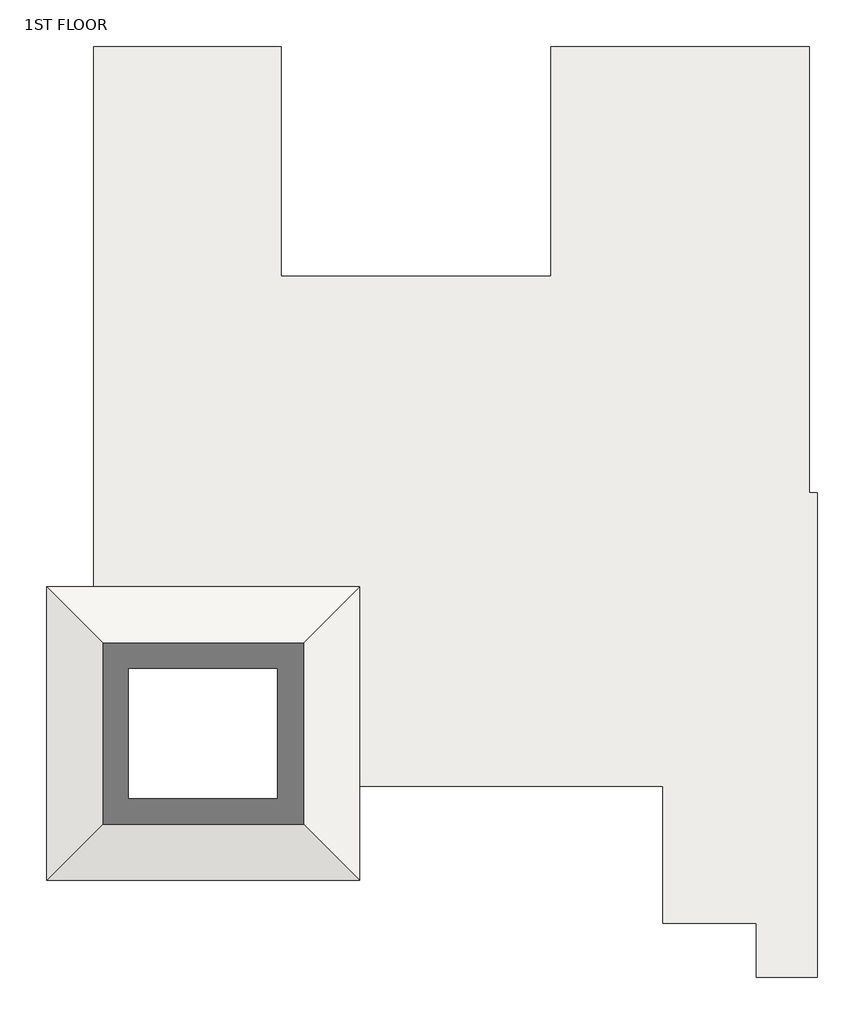
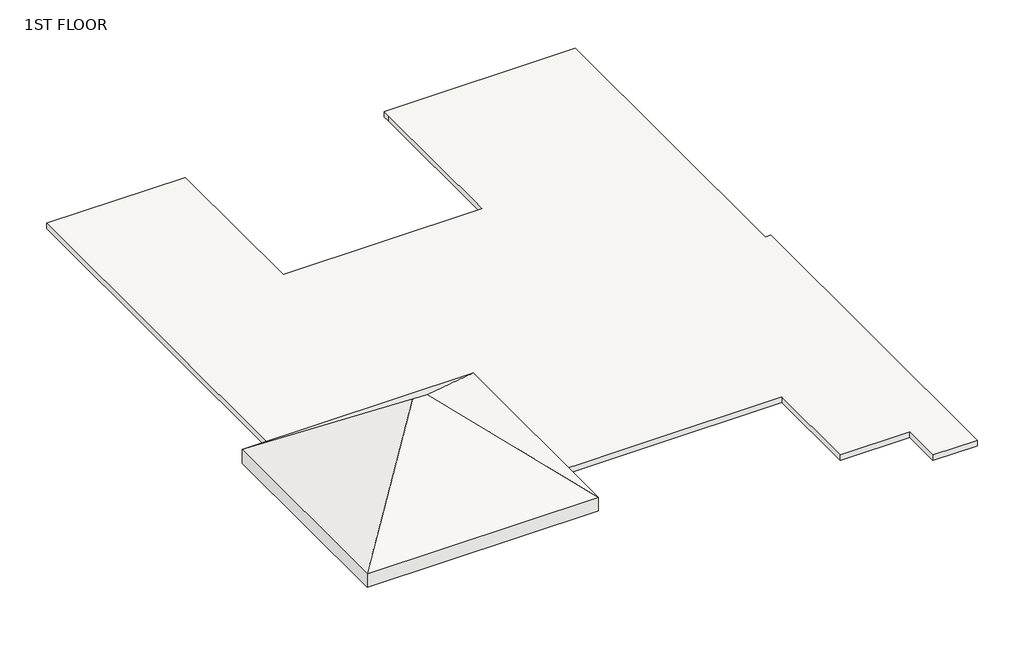
# One storey, incomplete: 1 roof, 1 slab.
"""IFC4 building model written with IfcOpenShell, lengths in millimetres."""

from ifc_helpers import new_model, si_unit, frame, origin, place, context, project, spatial, polyline, outline, extrude, faceted_brep, element, save

model = new_model("IFC4")

# Units and contexts
model_context = context("Model", 3, world=origin())
ifc_project = project(units=[si_unit("LENGTHUNIT", "METRE", prefix="MILLI")], contexts=[model_context])

# Site, building, storey
site = spatial("IfcSite", under=ifc_project)
building = spatial("IfcBuilding", under=site)
storey = spatial("IfcBuildingStorey", under=building, Name="1ST FLOOR", Elevation=4114.8)

# Roof
placement = place(None, origin())
element("IfcRoof", 1, ObjectType="Generic - 12\"", at=placement, inside=storey, context=model_context, shape_type="Brep", body=[
    faceted_brep([(473.5512825, 1161.1906886, 6257.925), (-2383.9487175, -1696.3093114, 4114.8), (-2383.9487175, 4018.6906886, 4114.8), (854.5512825, 1161.1906886, 6257.925), (3712.0512825, -1696.3093114, 4114.8), (3712.0512825, 4018.6906886, 4114.8), (-2383.9487175, -1696.3093114, 4495.8), (473.5512825, 1161.1906886, 6638.925), (-2383.9487175, 4018.6906886, 4495.8), (3712.0512825, -1696.3093114, 4495.8), (854.5512825, 1161.1906886, 6638.925), (3712.0512825, 4018.6906886, 4495.8)], [[[0, 1, 2]], [[1, 0, 3, 4]], [[4, 3, 5]], [[5, 3, 0, 2]], [[6, 7, 8]], [[6, 9, 10, 7]], [[9, 11, 10]], [[11, 8, 7, 10]], [[4, 9, 6, 1]], [[5, 11, 9, 4]], [[2, 8, 11, 5]], [[1, 6, 8, 2]]]),
])

# Slab
element("IfcSlab", 2, at=placement, inside=storey, context=model_context, shape_type="SweptSolid", body=[
    extrude(outline(polyline([(2188.0512825, 10063.8906886), (7445.8512825, 10063.8906886), (7445.8512825, 14331.0906886), (7445.8512825, 14534.2906886), (12475.0512825, 14534.2906886), (12475.0512825, 5847.4906886), (12627.4512825, 5847.4906886), (12627.4512825, -3588.6093114), (11446.3512825, -3588.6093114), (11446.3512825, -2534.5093114), (9617.5512825, -2534.5093114), (9617.5512825, 132.4906886), (2264.2512825, 132.4906886), (2264.2512825, 2189.8906886), (3712.0512825, 2189.8906886), (3712.0512825, 3180.4906886), (3102.4512825, 3180.4906886), (3102.4512825, 4018.6906886), (-1469.5487175, 4018.6906886), (-1469.5487175, 14534.2906886), (2188.0512825, 14534.2906886), (2188.0512825, 14305.6906886), (2188.0512825, 10063.8906886)])), frame((0.0, 0.0, 3962.4), z_axis=(0.0, 0.0, 1.0), x_axis=(1.0, 0.0, 0.0)), (0.0, 0.0, 1.0), 152.4),
])

save(model, "model.ifc")

# Revit data of these elements
# Type "Generic - 12\""
#   Assembly Code = "B1020"
#   Layers, outside or top first: 1' - 0" no material (function 1)
# Type
#   Assembly Code = "B1010"
#   Function = 0
#   Layers, outside or top first: 0' - 6" "Concrete, Cast-in-Place gray" (function 1)
# Element 1 (IfcRoof, "Generic - 12\"")
#   built-in parameter 1001705 = 21.7812 (stored number, unit not read)
#   built-in parameter 1001710 = 33615
#   Phase Created = New Construction
#   Materials on its faces: "Default Roof"
# Element 2 (IfcSlab)
#   Height Offset From Level = 0' - 0"
#   Phase Created = New Construction
#   Materials on its faces: "Concrete, Cast-in-Place gray"
# Materials
#   "Concrete, Cast-in-Place gray": class "Concrete", colour RGB 192 192 192, transparency 0, Description = "Cast-in-place concrete", Cost = 0
#   "Default Roof": colour RGB 88 101 114, transparency 0, Cost = 0
